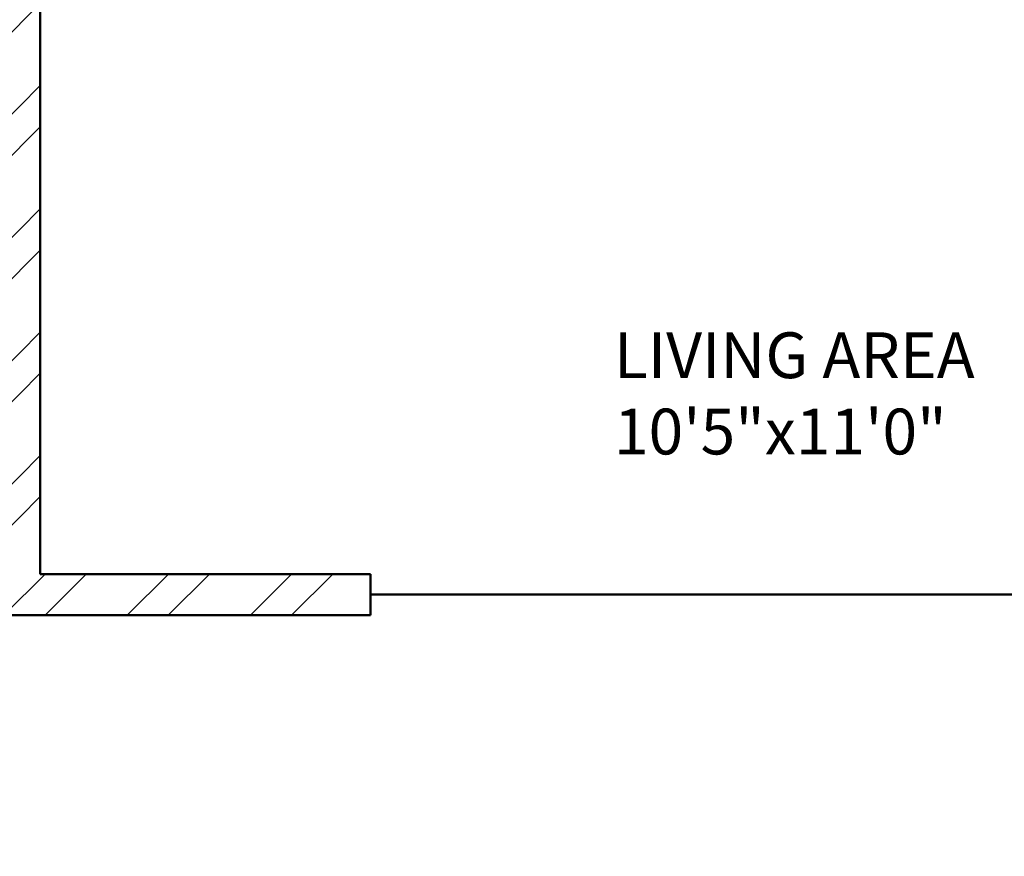
# Model space of a CAD drawing. Units: inches. Extents: x 1901 to 2863, y 888 to 2433.
# Tile 18 of 91: x 2157 to 2264, y 1549 to 1641. Entities that reach past the tile are written whole.
import ezdxf

# ---------------------------------------------------------------- set-up
doc = ezdxf.new("R2010")
doc.units = ezdxf.units.IN
for name, color, linetype, lineweight in [('A-AREA-IDEN', 7, 'Continuous', 18), ('A-WALL', 7, 'Continuous', 50), ('A-WALL-PATT', 8, 'Continuous', 13)]:
    doc.layers.add(name, color=color, linetype=linetype, lineweight=lineweight)
doc.styles.get("Standard").update_dxf_attribs({"font": 'arial.ttf'})

msp = doc.modelspace()

# ---------------------------------------------------------------- hatches: boundary and pattern name
at = {"layer": 'A-WALL-PATT'}
h = msp.add_hatch(dxfattribs=at)
h.set_pattern_fill('ANSI32', color=256)
h.paths.add_polyline_path([(2192.5, 2274.13), (2141.26, 2274.13), (2141.26, 2269.63), (2192.5, 2269.63)])
h.paths.add_polyline_path([(2259.93, 2274.13), (2216.5, 2274.13), (2216.5, 2269.63), (2255.43, 2269.63), (2255.43, 2214.63), (2250.81, 2214.63), (2250.81, 2210.13), (2259.93, 2210.13), (2259.93, 2215.13), (2271.76, 2215.13), (2271.76, 2217.38), (2271.76, 2219.63), (2259.93, 2219.63)])
h.paths.add_polyline_path([(2171.43, 2269.63), (2166.93, 2269.63), (2166.93, 2219.63), (2121.24, 2219.63), (2121.24, 2215.13), (2166.93, 2215.13), (2166.93, 2083.13), (2161.81, 2083.13), (2161.81, 2078.63), (2171.43, 2078.63), (2177, 2078.63), (2177, 2080.88), (2177, 2083.13), (2171.43, 2083.13), (2171.43, 2210.13), (2230.91, 2210.13), (2230.91, 2212.38), (2230.91, 2214.63), (2171.43, 2214.63)])
h.paths.add_polyline_path([(2117.26, 2274.13), (2089.43, 2274.13), (2089.43, 2219.63), (2081.14, 2219.63), (2081.14, 2215.13), (2089.43, 2215.13), (2098, 2215.13), (2098, 2217.38), (2098, 2219.63), (2093.93, 2219.63), (2093.93, 2269.63), (2117.26, 2269.63), (2117.26, 2271.88)])
h.paths.add_polyline_path([(2343.43, 2219.63), (2329.29, 2219.63), (2329.29, 2215.13), (2338.93, 2215.13), (2338.93, 2184.74), (2343.43, 2184.74)])
h.paths.add_polyline_path([(2338.93, 2083.13), (2329.29, 2083.13), (2208.97, 2083.13), (2208.97, 2078.63), (2338.93, 2078.63)])
h.paths.add_polyline_path([(2343.43, 2136.74), (2338.93, 2136.74), (2338.93, 1872.63), (2343.43, 1872.63)])
h.paths.add_polyline_path([(2343.43, 1863.63), (2397.68, 1863.63), (2397.68, 1821.63), (2384.14, 1821.63), (2384.14, 1812.63), (2418.33, 1812.63), (2418.33, 1817.13), (2418.33, 1821.63), (2406.68, 1821.63), (2406.68, 1863.63), (2459.5, 1863.63), (2459.5, 1821.63), (2447.14, 1821.63), (2447.14, 1812.63), (2459.5, 1812.63), (2468.5, 1812.63), (2468.5, 1872.63), (2394.43, 1872.63), (2334.43, 1872.63), (2334.43, 1812.63), (2343.43, 1812.63), (2353.25, 1812.63), (2353.25, 1821.63), (2343.43, 1821.63)])
h.paths.add_polyline_path([(2510.01, 1872.63), (2468.5, 1872.63), (2468.5, 1868.13), (2510.01, 1868.13)])
h.paths.add_polyline_path([(2514.01, 1817.13), (2468.5, 1817.13), (2468.5, 1812.63), (2482.11, 1812.63), (2482.11, 1800.61), (2486.61, 1800.61), (2486.61, 1812.63), (2514.01, 1812.63)])
h.paths.add_polyline_path([(2299.25, 1814.88), (2299.25, 1817.13), (2295.93, 1817.13), (2295.93, 1854.17), (2293.68, 1854.17), (2291.43, 1854.17), (2291.43, 1817.13), (2266.11, 1817.13), (2266.11, 1812.63), (2299.25, 1812.63)])
h.paths.add_polyline_path([(2218.11, 1817.13), (2206.46, 1817.13), (2171.43, 1817.13), (2171.43, 1949.13), (2190.1, 1949.13), (2190.1, 1953.63), (2163.47, 1953.63), (2163.47, 1949.13), (2166.93, 1949.13), (2166.93, 1817.13), (2114.3, 1817.13), (2114.3, 1812.63), (2218.11, 1812.63)])
h.paths.add_polyline_path([(2029.43, 1970.92), (2024.93, 1970.92), (2024.93, 1912.72), (2029.43, 1912.72)])
h.paths.add_polyline_path([(2132.3, 1953.63), (2113.93, 1953.63), (2113.93, 1975.89), (2111.68, 1975.89), (2109.43, 1975.89), (2109.43, 1953.63), (2029.43, 1953.63), (2029.43, 1949.13), (2132.3, 1949.13)])
h.paths.add_polyline_path([(2029.43, 1853.61), (2029.31, 1853.61), (2029.31, 1853.61), (2029.43, 1853.61), (2029.43, 1864.72), (2024.93, 1864.72), (2024.93, 1812.63), (2066.3, 1812.63), (2066.3, 1814.88), (2066.3, 1817.13), (2029.43, 1817.13)])
h.paths.add_polyline_path([(2122.93, 2010.09), (2120.68, 2010.09), (2118.43, 2010.09), (2118.43, 2006.13), (2029.43, 2006.13), (2029.43, 2001.63), (2109.43, 2001.63), (2109.43, 1998.04), (2113.93, 1998.04), (2113.93, 2001.63), (2122.93, 2001.63)])
h.paths.add_polyline_path([(2029.43, 2031.38), (2024.93, 2031.38), (2024.93, 1994.92), (2027.18, 1994.92), (2029.43, 1994.92)])
h.paths.add_polyline_path([(2029.43, 2136.74), (2024.93, 2136.74), (2024.93, 2067.38), (2027.18, 2067.38), (2029.43, 2067.38)])
h.paths.add_polyline_path([(2125.62, 2083.13), (2029.43, 2083.13), (2029.43, 2078.63), (2118.43, 2078.63), (2118.43, 2030.71), (2122.93, 2030.71), (2122.93, 2078.63), (2125.62, 2078.63)])
h.paths.add_polyline_path([(2029.43, 2215.13), (2040.47, 2215.13), (2040.47, 2217.38), (2040.47, 2219.63), (2024.93, 2219.63), (2024.93, 2184.74), (2029.43, 2184.74), (2029.43, 2187.78)])
h.paths.add_polyline_path([(2686.43, 2274.13), (2659.28, 2274.13), (2659.28, 2269.63), (2681.93, 2269.63), (2681.93, 2219.63), (2676.82, 2219.63), (2676.82, 2215.13), (2681.93, 2215.13), (2697.01, 2215.13), (2697.01, 2217.38), (2697.01, 2219.63), (2686.43, 2219.63)])
h.paths.add_polyline_path([(2609.93, 2269.63), (2635.28, 2269.63), (2635.28, 2274.13), (2571.43, 2274.13), (2571.43, 2269.63), (2605.43, 2269.63), (2605.43, 2214.63), (2549.1, 2214.63), (2549.1, 2210.13), (2605.43, 2210.13), (2605.43, 2083.13), (2601.01, 2083.13), (2601.01, 2080.88), (2601.01, 2078.63), (2609.93, 2078.63), (2616.16, 2078.63), (2616.16, 2080.88), (2616.16, 2083.13), (2609.93, 2083.13), (2609.93, 2215.13), (2651.46, 2215.13), (2651.46, 2217.38), (2651.46, 2219.63), (2609.93, 2219.63)])
h.paths.add_polyline_path([(2521.43, 2269.63), (2547.43, 2269.63), (2547.43, 2271.88), (2547.43, 2274.13), (2516.93, 2274.13), (2516.93, 2219.63), (2506.41, 2219.63), (2506.41, 2215.13), (2516.93, 2215.13), (2516.93, 2210.13), (2525.4, 2210.13), (2525.4, 2212.38), (2525.4, 2214.63), (2521.43, 2214.63)])
h.paths.add_polyline_path([(2456.01, 2219.63), (2439.43, 2219.63), (2439.43, 2187.89), (2443.93, 2187.89), (2443.93, 2215.13), (2456.01, 2215.13)])
h.paths.add_polyline_path([(2752.93, 2219.63), (2739.48, 2219.63), (2739.48, 2215.13), (2748.43, 2215.13), (2748.43, 2187.89), (2752.93, 2187.89)])
h.paths.add_polyline_path([(2752.93, 2139.89), (2748.43, 2139.89), (2748.43, 2083.13), (2648.42, 2083.13), (2648.42, 2078.63), (2654.93, 2078.63), (2654.93, 2039.44), (2659.43, 2039.44), (2659.43, 2078.63), (2748.43, 2078.63), (2748.43, 2063.43), (2752.93, 2063.43)])
h.paths.add_polyline_path([(2752.93, 2010.63), (2659.43, 2010.63), (2659.43, 2015.65), (2654.93, 2015.65), (2654.93, 2010.63), (2605.43, 2010.63), (2605.43, 1920.97), (2609.93, 1920.97), (2609.93, 2006.13), (2748.43, 2006.13), (2748.43, 1982.47), (2752.93, 1982.47)])
h.paths.add_polyline_path([(2752.93, 2027.43), (2748.43, 2027.43), (2748.43, 2010.63), (2752.93, 2010.63)])
h.paths.add_polyline_path([(2748.43, 1886.13), (2609.93, 1886.13), (2609.93, 1889.72), (2605.43, 1889.72), (2605.43, 1861.26), (2609.93, 1861.26), (2609.93, 1881.63), (2748.43, 1881.63)])
h.paths.add_polyline_path([(2456.86, 2228.83), (2498.4, 2228.83), (2498.4, 2247.49), (2456.86, 2247.49)], flags=9)
h.paths.add_polyline_path([(2038.6, 2237.42), (2080.17, 2237.42), (2080.17, 2256.08), (2038.6, 2256.08)], flags=9)
h.paths.add_polyline_path([(2292.01, 1062.39), (2539.93, 1062.39), (2539.93, 1099.49), (2292.01, 1099.49)], flags=9)
h.paths.add_polyline_path([(2424.91, 1832.25), (2448.51, 1832.25), (2448.51, 1846.68), (2424.91, 1846.68)], flags=25)
h.paths.add_polyline_path([(2359.08, 1832.25), (2382.68, 1832.25), (2382.68, 1846.68), (2359.08, 1846.68)], flags=25)
h.paths.add_polyline_path([(2352.9, 1684.8), (2367.54, 1684.8), (2367.54, 1697.17), (2352.9, 1697.17)], flags=9)
h.paths.add_polyline_path([(2079.29, 1755.83), (2169.02, 1755.83), (2169.02, 1774.37), (2079.29, 1774.37)], flags=9)
h.paths.add_polyline_path([(2404.09, 1373.86), (2404.09, 1463.59), (2385.54, 1463.59), (2385.54, 1373.86)], flags=9)
h.paths.add_polyline_path([(2268.09, 2236.37), (2309.64, 2236.37), (2309.64, 2255.03), (2268.09, 2255.03)], flags=9)
h.paths.add_polyline_path([(2575.96, 1700.95), (2665.7, 1700.95), (2665.7, 1719.5), (2575.96, 1719.5)], flags=9)
h.paths.add_polyline_path([(2302.96, 1878.47), (2329.52, 1878.47), (2329.52, 1888.78), (2302.96, 1888.78)], flags=9)
h.paths.add_polyline_path([(2097.42, 2240.58), (2126.57, 2240.58), (2126.57, 2259.23), (2097.42, 2259.23)], flags=9)
h.paths.add_polyline_path([(2208.72, 2246.12), (2237.88, 2246.12), (2237.88, 2264.78), (2208.72, 2264.78)], flags=9)
h.paths.add_polyline_path([(2038.15, 1925.96), (2076.99, 1925.96), (2076.99, 1944.62), (2038.15, 1944.62)], flags=9)
h.paths.add_polyline_path([(2239.14, 1926.67), (2288.46, 1926.67), (2288.46, 1945.33), (2239.14, 1945.33)], flags=9)
h.paths.add_polyline_path([(2175.43, 2007.33), (2212.36, 2007.33), (2212.36, 2025.99), (2175.43, 2025.99)], flags=9)
h.paths.add_polyline_path([(2225.03, 2091.79), (2263.87, 2091.79), (2263.87, 2110.45), (2225.03, 2110.45)], flags=9)
h.paths.add_polyline_path([(2035.4, 2098.48), (2074.24, 2098.48), (2074.24, 2117.14), (2035.4, 2117.14)], flags=9)
h.paths.add_polyline_path([(2050.1, 2029.21), (2083.26, 2029.21), (2083.26, 2047.87), (2050.1, 2047.87)], flags=9)
h.paths.add_polyline_path([(2069.68, 1956.72), (2098.83, 1956.72), (2098.83, 1975.38), (2069.68, 1975.38)], flags=25)
h.paths.add_polyline_path([(2328.62, 1753.34), (2361.66, 1753.34), (2361.66, 1771.99), (2328.62, 1771.99)], flags=9)
h.paths.add_polyline_path([(2395.16, 2060.89), (2395.16, 2140.65), (2378.68, 2140.65), (2378.68, 2060.89)], flags=9)
h.paths.add_polyline_path([(2463.73, 2059.02), (2492.89, 2059.02), (2492.89, 2077.68), (2463.73, 2077.68)], flags=9)
h.paths.add_polyline_path([(2458.03, 2181.54), (2496.87, 2181.54), (2496.87, 2200.19), (2458.03, 2200.19)], flags=9)
h.paths.add_polyline_path([(2527.58, 2243.07), (2556.73, 2243.07), (2556.73, 2261.73), (2527.58, 2261.73)], flags=9)
h.paths.add_polyline_path([(2694.46, 2232.77), (2736.03, 2232.77), (2736.03, 2251.42), (2694.46, 2251.42)], flags=9)
h.paths.add_polyline_path([(2637.82, 2249.22), (2666.98, 2249.22), (2666.98, 2267.88), (2637.82, 2267.88)], flags=9)
h.paths.add_polyline_path([(2623.69, 2183.54), (2662.53, 2183.54), (2662.53, 2202.2), (2623.69, 2202.2)], flags=9)
h.paths.add_polyline_path([(2691.97, 2021.5), (2725.12, 2021.5), (2725.12, 2040.16), (2691.97, 2040.16)], flags=9)
h.paths.add_polyline_path([(2621.04, 1975.91), (2662.34, 1975.91), (2662.34, 1994.57), (2621.04, 1994.57)], flags=25)
h.paths.add_polyline_path([(2479.03, 1927.62), (2519.84, 1927.62), (2519.84, 1946.28), (2479.03, 1946.28)], flags=9)
h.paths.add_polyline_path([(2670.94, 1849.08), (2716.01, 1849.08), (2716.01, 1867.73), (2670.94, 1867.73)], flags=9)
h.paths.add_polyline_path([(2523.61, 1782.96), (2550.17, 1782.96), (2550.17, 1793.26), (2523.61, 1793.26)], flags=9)
h.paths.add_polyline_path([(2450.84, 1207.33), (2492.39, 1207.33), (2492.39, 1225.99), (2450.84, 1225.99)], flags=9)
h.paths.add_polyline_path([(2527.75, 1203.84), (2556.91, 1203.84), (2556.91, 1222.5), (2527.75, 1222.5)], flags=9)
h.paths.add_polyline_path([(2639.11, 1207.2), (2668.27, 1207.2), (2668.27, 1225.86), (2639.11, 1225.86)], flags=9)
h.paths.add_polyline_path([(2692.59, 1218.97), (2734.17, 1218.97), (2734.17, 1237.62), (2692.59, 1237.62)], flags=9)
h.paths.add_polyline_path([(2669.27, 1366.33), (2708.11, 1366.33), (2708.11, 1384.99), (2669.27, 1384.99)], flags=9)
h.paths.add_polyline_path([(2463.31, 1358.03), (2502.15, 1358.03), (2502.15, 1376.69), (2463.31, 1376.69)], flags=9)
h.paths.add_polyline_path([(2494.72, 1449.96), (2531.65, 1449.96), (2531.65, 1468.62), (2494.72, 1468.62)], flags=9)
h.paths.add_polyline_path([(2675.57, 1422.16), (2708.72, 1422.16), (2708.72, 1440.81), (2675.57, 1440.81)], flags=9)
h.paths.add_polyline_path([(2685.63, 1493.89), (2714.79, 1493.89), (2714.79, 1512.55), (2685.63, 1512.55)], flags=9)
h.paths.add_polyline_path([(2686.8, 1529.91), (2725.65, 1529.91), (2725.65, 1548.57), (2686.8, 1548.57)], flags=9)
h.paths.add_polyline_path([(2503.65, 1537.99), (2552.97, 1537.99), (2552.97, 1556.65), (2503.65, 1556.65)], flags=9)
h.paths.add_polyline_path([(2291.71, 1643.5), (2318.28, 1643.5), (2318.28, 1653.81), (2291.71, 1653.81)], flags=9)
h.paths.add_polyline_path([(2450.63, 1610.52), (2477.19, 1610.52), (2477.19, 1620.82), (2450.63, 1620.82)], flags=9)
h.paths.add_polyline_path([(2359.99, 1551.81), (2422.25, 1551.81), (2422.25, 1562.12), (2359.99, 1562.12)], flags=9)
h.paths.add_polyline_path([(2280.11, 1249.01), (2321.65, 1249.01), (2321.65, 1267.66), (2280.11, 1267.66)], flags=9)
h.paths.add_polyline_path([(2164.06, 1274.23), (2193.22, 1274.23), (2193.22, 1292.89), (2164.06, 1292.89)], flags=9)
h.paths.add_polyline_path([(2118.21, 1277.69), (2151.25, 1277.69), (2151.25, 1296.35), (2118.21, 1296.35)], flags=9)
h.paths.add_polyline_path([(2031.95, 1268.53), (2073.52, 1268.53), (2073.52, 1287.19), (2031.95, 1287.19)], flags=9)
h.paths.add_polyline_path([(2050.2, 1409.08), (2089.04, 1409.08), (2089.04, 1427.74), (2050.2, 1427.74)], flags=9)
h.paths.add_polyline_path([(2243.74, 1421.03), (2282.58, 1421.03), (2282.58, 1439.69), (2243.74, 1439.69)], flags=9)
h.paths.add_polyline_path([(2190.75, 1509.77), (2231.56, 1509.77), (2231.56, 1528.43), (2190.75, 1528.43)], flags=9)
h.paths.add_polyline_path([(2058.39, 1475.42), (2091.55, 1475.42), (2091.55, 1494.07), (2058.39, 1494.07)], flags=9)
h.paths.add_polyline_path([(2062.45, 1553.09), (2091.6, 1553.09), (2091.6, 1571.75), (2062.45, 1571.75)], flags=9)
h.paths.add_polyline_path([(2219.52, 1590.37), (2266.15, 1590.37), (2266.15, 1609.02), (2219.52, 1609.02)], flags=9)
h.paths.add_polyline_path([(2041.07, 1584.19), (2079.91, 1584.19), (2079.91, 1602.85), (2041.07, 1602.85)], flags=9)
h = msp.add_hatch(dxfattribs=at)
h.set_pattern_fill('ANSI32', color=256)
h.paths.add_polyline_path([(2443.93, 2139.89), (2439.43, 2139.89), (2439.43, 2069.35), (2441.68, 2069.35), (2443.93, 2069.35), (2443.93, 2078.63), (2521.93, 2078.63), (2521.93, 2075.07), (2524.18, 2075.07), (2526.43, 2075.07), (2526.43, 2078.63), (2571.75, 2078.63), (2571.75, 2080.88), (2571.75, 2083.13), (2443.93, 2083.13)])
h.paths.add_polyline_path([(2526.43, 2054.63), (2524.18, 2054.63), (2521.93, 2054.63), (2521.93, 2030.63), (2443.93, 2030.63), (2443.93, 2045.35), (2439.43, 2045.35), (2439.43, 1983.87), (2443.93, 1983.87), (2443.93, 2026.13), (2521.93, 2026.13), (2526.43, 2026.13)])
h.paths.add_polyline_path([(2443.93, 1923.87), (2439.43, 1923.87), (2439.43, 1872.63), (2443.93, 1872.63)])
h.paths.add_polyline_path([(2636.23, 1766.13), (2609.93, 1766.13), (2609.93, 1779.79), (2605.43, 1779.79), (2605.43, 1766.13), (2486.61, 1766.13), (2486.61, 1770.67), (2482.11, 1770.67), (2482.11, 1766.13), (2482.11, 1761.63), (2636.23, 1761.63), (2636.23, 1763.88)])
h.paths.add_polyline_path([(2519.54, 1663.38), (2519.54, 1665.63), (2494.93, 1665.63), (2481.83, 1665.63), (2481.83, 1663.38), (2481.83, 1661.13), (2490.43, 1661.13), (2490.43, 1640.16), (2494.93, 1640.16), (2494.93, 1661.13), (2519.54, 1661.13)])
h.paths.add_polyline_path([(2443.93, 1712.13), (2443.93, 1716.63), (2414.46, 1716.63), (2414.46, 1712.13), (2439.43, 1712.13), (2439.43, 1545.51), (2443.93, 1545.51), (2443.93, 1661.13), (2448.47, 1661.13), (2448.47, 1665.63), (2443.93, 1665.63)])
h.paths.add_polyline_path([(2343.43, 1712.13), (2365.52, 1712.13), (2365.52, 1714.38), (2365.52, 1716.63), (2333.87, 1716.63), (2333.87, 1714.38), (2333.87, 1712.13), (2338.93, 1712.13), (2338.93, 1575.63), (2338.93, 1545.51), (2343.43, 1545.51), (2343.43, 1547.51), (2343.43, 1580.13)])
h.paths.add_polyline_path([(2752.93, 1665.63), (2579.54, 1665.63), (2579.54, 1661.13), (2615.93, 1661.13), (2615.93, 1529.13), (2598.93, 1529.13), (2598.93, 1524.63), (2623.13, 1524.63), (2623.13, 1526.88), (2623.13, 1529.13), (2620.43, 1529.13), (2620.43, 1661.13), (2748.43, 1661.13), (2748.43, 1633.5), (2752.93, 1633.5)])
h.paths.add_polyline_path([(2752.93, 1419.93), (2748.43, 1419.93), (2748.43, 1400.13), (2659.43, 1400.13), (2659.43, 1444.33), (2657.18, 1444.33), (2654.93, 1444.33), (2654.93, 1400.13), (2643.65, 1400.13), (2643.65, 1395.63), (2748.43, 1395.63), (2748.43, 1364.04), (2752.93, 1364.04)])
h.paths.add_polyline_path([(2752.93, 1492.88), (2748.43, 1492.88), (2748.43, 1476.63), (2667.43, 1476.63), (2667.43, 1479.71), (2665.18, 1479.71), (2662.93, 1479.71), (2662.93, 1476.63), (2654.93, 1476.63), (2654.93, 1469.54), (2659.43, 1469.54), (2659.43, 1472.13), (2748.43, 1472.13), (2748.43, 1455.93), (2752.93, 1455.93)])
h.paths.add_polyline_path([(2752.93, 1304.04), (2748.43, 1304.04), (2748.43, 1263.63), (2738.66, 1263.63), (2738.66, 1259.13), (2752.93, 1259.13)])
h.paths.add_polyline_path([(2685.93, 1259.13), (2695.49, 1259.13), (2695.49, 1261.38), (2695.49, 1263.63), (2677.84, 1263.63), (2677.84, 1261.38), (2677.84, 1259.13), (2681.43, 1259.13), (2681.43, 1203.63), (2653.28, 1203.63), (2653.28, 1199.13), (2685.93, 1199.13), (2685.93, 1203.63)])
h.paths.add_polyline_path([(2609.43, 1395.63), (2611.85, 1395.63), (2611.85, 1400.13), (2598.89, 1400.13), (2598.89, 1397.88), (2598.89, 1395.63), (2604.93, 1395.63), (2604.93, 1268.13), (2554.73, 1268.13), (2554.73, 1265.88), (2554.73, 1263.63), (2604.93, 1263.63), (2604.93, 1203.63), (2571.31, 1203.63), (2571.31, 1199.13), (2604.93, 1199.13), (2629.28, 1199.13), (2629.28, 1201.38), (2629.28, 1203.63), (2609.43, 1203.63), (2609.43, 1258.63), (2609.43, 1259.13), (2654.8, 1259.13), (2654.8, 1263.63), (2609.43, 1263.63)])
h.paths.add_polyline_path([(2443.93, 1304.04), (2439.43, 1304.04), (2439.43, 1259.13), (2443.93, 1259.13), (2456.16, 1259.13), (2456.16, 1261.38), (2456.16, 1263.63), (2443.93, 1263.63)])
h.paths.add_polyline_path([(2525.43, 1263.63), (2531.78, 1263.63), (2531.78, 1268.13), (2520.93, 1268.13), (2520.93, 1263.63), (2511.41, 1263.63), (2511.41, 1259.13), (2520.93, 1259.13), (2520.93, 1199.13), (2547.31, 1199.13), (2547.31, 1201.38), (2547.31, 1203.63), (2525.43, 1203.63)])
h.paths.add_polyline_path([(2443.93, 1434.84), (2439.43, 1434.84), (2439.43, 1364.04), (2441.68, 1364.04), (2443.93, 1364.04)])
h.paths.add_polyline_path([(2567.13, 1400.13), (2443.93, 1400.13), (2443.93, 1395.63), (2567.13, 1395.63)])
h.paths.add_polyline_path([(2443.93, 1545.51), (2439.43, 1545.51), (2439.43, 1494.84), (2443.93, 1494.84)])
h.paths.add_polyline_path([(2494.93, 1553.35), (2492.68, 1553.35), (2490.43, 1553.35), (2490.43, 1524.63), (2494.93, 1524.63), (2525.94, 1524.63), (2525.94, 1526.88), (2525.94, 1529.13), (2494.93, 1529.13)])
h.paths.add_polyline_path([(2752.93, 1573.5), (2748.43, 1573.5), (2748.43, 1529.13), (2657.76, 1529.13), (2657.76, 1524.63), (2662.93, 1524.63), (2662.93, 1498.63), (2667.43, 1498.63), (2667.43, 1524.63), (2748.43, 1524.63), (2748.43, 1516.88), (2752.93, 1516.88)])
h.paths.add_polyline_path([(2038.6, 2237.42), (2080.17, 2237.42), (2080.17, 2256.08), (2038.6, 2256.08)], flags=9)
h.paths.add_polyline_path([(2292.01, 1062.39), (2539.93, 1062.39), (2539.93, 1099.49), (2292.01, 1099.49)], flags=9)
h.paths.add_polyline_path([(2424.91, 1832.25), (2448.51, 1832.25), (2448.51, 1846.68), (2424.91, 1846.68)], flags=9)
h.paths.add_polyline_path([(2359.08, 1832.25), (2382.68, 1832.25), (2382.68, 1846.68), (2359.08, 1846.68)], flags=9)
h.paths.add_polyline_path([(2352.9, 1684.8), (2367.54, 1684.8), (2367.54, 1697.17), (2352.9, 1697.17)], flags=9)
h.paths.add_polyline_path([(2079.29, 1755.83), (2169.02, 1755.83), (2169.02, 1774.37), (2079.29, 1774.37)], flags=9)
h.paths.add_polyline_path([(2404.09, 1373.86), (2404.09, 1463.59), (2385.54, 1463.59), (2385.54, 1373.86)], flags=9)
h.paths.add_polyline_path([(2268.09, 2236.37), (2309.64, 2236.37), (2309.64, 2255.03), (2268.09, 2255.03)], flags=9)
h.paths.add_polyline_path([(2575.96, 1700.95), (2665.7, 1700.95), (2665.7, 1719.5), (2575.96, 1719.5)], flags=9)
h.paths.add_polyline_path([(2302.96, 1878.47), (2329.52, 1878.47), (2329.52, 1888.78), (2302.96, 1888.78)], flags=9)
h.paths.add_polyline_path([(2097.42, 2240.58), (2126.57, 2240.58), (2126.57, 2259.23), (2097.42, 2259.23)], flags=9)
h.paths.add_polyline_path([(2208.72, 2246.12), (2237.88, 2246.12), (2237.88, 2264.78), (2208.72, 2264.78)], flags=9)
h.paths.add_polyline_path([(2038.15, 1925.96), (2076.99, 1925.96), (2076.99, 1944.62), (2038.15, 1944.62)], flags=9)
h.paths.add_polyline_path([(2239.14, 1926.67), (2288.46, 1926.67), (2288.46, 1945.33), (2239.14, 1945.33)], flags=9)
h.paths.add_polyline_path([(2175.43, 2007.33), (2212.36, 2007.33), (2212.36, 2025.99), (2175.43, 2025.99)], flags=9)
h.paths.add_polyline_path([(2225.03, 2091.79), (2263.87, 2091.79), (2263.87, 2110.45), (2225.03, 2110.45)], flags=9)
h.paths.add_polyline_path([(2035.4, 2098.48), (2074.24, 2098.48), (2074.24, 2117.14), (2035.4, 2117.14)], flags=9)
h.paths.add_polyline_path([(2050.1, 2029.21), (2083.26, 2029.21), (2083.26, 2047.87), (2050.1, 2047.87)], flags=9)
h.paths.add_polyline_path([(2069.68, 1956.72), (2098.83, 1956.72), (2098.83, 1975.38), (2069.68, 1975.38)], flags=9)
h.paths.add_polyline_path([(2328.62, 1753.34), (2361.66, 1753.34), (2361.66, 1771.99), (2328.62, 1771.99)], flags=9)
h.paths.add_polyline_path([(2395.16, 2060.89), (2395.16, 2140.65), (2378.68, 2140.65), (2378.68, 2060.89)], flags=9)
h.paths.add_polyline_path([(2463.73, 2059.02), (2492.89, 2059.02), (2492.89, 2077.68), (2463.73, 2077.68)], flags=9)
h.paths.add_polyline_path([(2458.03, 2181.54), (2496.87, 2181.54), (2496.87, 2200.19), (2458.03, 2200.19)], flags=9)
h.paths.add_polyline_path([(2456.86, 2228.83), (2498.4, 2228.83), (2498.4, 2247.49), (2456.86, 2247.49)], flags=9)
h.paths.add_polyline_path([(2527.58, 2243.07), (2556.73, 2243.07), (2556.73, 2261.73), (2527.58, 2261.73)], flags=9)
h.paths.add_polyline_path([(2694.46, 2232.77), (2736.03, 2232.77), (2736.03, 2251.42), (2694.46, 2251.42)], flags=9)
h.paths.add_polyline_path([(2637.82, 2249.22), (2666.98, 2249.22), (2666.98, 2267.88), (2637.82, 2267.88)], flags=9)
h.paths.add_polyline_path([(2623.69, 2183.54), (2662.53, 2183.54), (2662.53, 2202.2), (2623.69, 2202.2)], flags=9)
h.paths.add_polyline_path([(2691.97, 2021.5), (2725.12, 2021.5), (2725.12, 2040.16), (2691.97, 2040.16)], flags=9)
h.paths.add_polyline_path([(2621.04, 1975.91), (2662.34, 1975.91), (2662.34, 1994.57), (2621.04, 1994.57)], flags=9)
h.paths.add_polyline_path([(2479.03, 1927.62), (2519.84, 1927.62), (2519.84, 1946.28), (2479.03, 1946.28)], flags=9)
h.paths.add_polyline_path([(2670.94, 1849.08), (2716.01, 1849.08), (2716.01, 1867.73), (2670.94, 1867.73)], flags=9)
h.paths.add_polyline_path([(2523.61, 1782.96), (2550.17, 1782.96), (2550.17, 1793.26), (2523.61, 1793.26)], flags=9)
h.paths.add_polyline_path([(2450.84, 1207.33), (2492.39, 1207.33), (2492.39, 1225.99), (2450.84, 1225.99)], flags=9)
h.paths.add_polyline_path([(2527.75, 1203.84), (2556.91, 1203.84), (2556.91, 1222.5), (2527.75, 1222.5)], flags=9)
h.paths.add_polyline_path([(2639.11, 1207.2), (2668.27, 1207.2), (2668.27, 1225.86), (2639.11, 1225.86)], flags=9)
h.paths.add_polyline_path([(2692.59, 1218.97), (2734.17, 1218.97), (2734.17, 1237.62), (2692.59, 1237.62)], flags=9)
h.paths.add_polyline_path([(2669.27, 1366.33), (2708.11, 1366.33), (2708.11, 1384.99), (2669.27, 1384.99)], flags=25)
h.paths.add_polyline_path([(2463.31, 1358.03), (2502.15, 1358.03), (2502.15, 1376.69), (2463.31, 1376.69)], flags=9)
h.paths.add_polyline_path([(2494.72, 1449.96), (2531.65, 1449.96), (2531.65, 1468.62), (2494.72, 1468.62)], flags=9)
h.paths.add_polyline_path([(2675.57, 1422.16), (2708.72, 1422.16), (2708.72, 1440.81), (2675.57, 1440.81)], flags=25)
h.paths.add_polyline_path([(2685.63, 1493.89), (2714.79, 1493.89), (2714.79, 1512.55), (2685.63, 1512.55)], flags=9)
h.paths.add_polyline_path([(2686.8, 1529.91), (2725.65, 1529.91), (2725.65, 1548.57), (2686.8, 1548.57)], flags=25)
h.paths.add_polyline_path([(2503.65, 1537.99), (2552.97, 1537.99), (2552.97, 1556.65), (2503.65, 1556.65)], flags=9)
h.paths.add_polyline_path([(2291.71, 1643.5), (2318.28, 1643.5), (2318.28, 1653.81), (2291.71, 1653.81)], flags=9)
h.paths.add_polyline_path([(2450.63, 1610.52), (2477.19, 1610.52), (2477.19, 1620.82), (2450.63, 1620.82)], flags=9)
h.paths.add_polyline_path([(2359.99, 1551.81), (2422.25, 1551.81), (2422.25, 1562.12), (2359.99, 1562.12)], flags=9)
h.paths.add_polyline_path([(2280.11, 1249.01), (2321.65, 1249.01), (2321.65, 1267.66), (2280.11, 1267.66)], flags=9)
h.paths.add_polyline_path([(2164.06, 1274.23), (2193.22, 1274.23), (2193.22, 1292.89), (2164.06, 1292.89)], flags=9)
h.paths.add_polyline_path([(2118.21, 1277.69), (2151.25, 1277.69), (2151.25, 1296.35), (2118.21, 1296.35)], flags=9)
h.paths.add_polyline_path([(2031.95, 1268.53), (2073.52, 1268.53), (2073.52, 1287.19), (2031.95, 1287.19)], flags=9)
h.paths.add_polyline_path([(2050.2, 1409.08), (2089.04, 1409.08), (2089.04, 1427.74), (2050.2, 1427.74)], flags=9)
h.paths.add_polyline_path([(2243.74, 1421.03), (2282.58, 1421.03), (2282.58, 1439.69), (2243.74, 1439.69)], flags=9)
h.paths.add_polyline_path([(2190.75, 1509.77), (2231.56, 1509.77), (2231.56, 1528.43), (2190.75, 1528.43)], flags=9)
h.paths.add_polyline_path([(2058.39, 1475.42), (2091.55, 1475.42), (2091.55, 1494.07), (2058.39, 1494.07)], flags=9)
h.paths.add_polyline_path([(2062.45, 1553.09), (2091.6, 1553.09), (2091.6, 1571.75), (2062.45, 1571.75)], flags=9)
h.paths.add_polyline_path([(2219.52, 1590.37), (2266.15, 1590.37), (2266.15, 1609.02), (2219.52, 1609.02)], flags=9)
h.paths.add_polyline_path([(2041.07, 1584.19), (2079.91, 1584.19), (2079.91, 1602.85), (2041.07, 1602.85)], flags=9)
h = msp.add_hatch(dxfattribs=at)
h.set_pattern_fill('ANSI32', color=256)
h.paths.add_polyline_path([(2182.93, 1716.63), (2024.93, 1716.63), (2024.93, 1681.7), (2029.33, 1681.7), (2029.33, 1712.13), (2154.33, 1712.13), (2154.33, 1580.13), (2148.52, 1580.13), (2148.52, 1577.88), (2148.52, 1575.63), (2194.93, 1575.63), (2194.93, 1580.13), (2158.83, 1580.13), (2158.83, 1712.13), (2182.93, 1712.13)])
h.paths.add_polyline_path([(2301.07, 1716.63), (2242.93, 1716.63), (2242.93, 1712.13), (2283.83, 1712.13), (2283.83, 1685.54), (2288.33, 1685.54), (2288.33, 1712.13), (2301.07, 1712.13)])
h.paths.add_polyline_path([(2288.33, 1600.41), (2286.08, 1600.41), (2283.83, 1600.41), (2283.83, 1580.13), (2270.6, 1580.13), (2270.6, 1575.63), (2288.33, 1575.63)])
h.paths.add_polyline_path([(2295.93, 1953.63), (2271.45, 1953.63), (2271.45, 1949.13), (2291.43, 1949.13), (2291.43, 1941.24), (2295.93, 1941.24)])
h.paths.add_polyline_path([(2098.38, 1244.13), (2082.33, 1244.13), (2082.33, 1302.13), (2086.52, 1302.13), (2086.52, 1306.63), (2067.46, 1306.63), (2067.46, 1302.13), (2077.83, 1302.13), (2077.83, 1239.63), (2098.38, 1239.63), (2098.38, 1241.88)])
h.paths.add_polyline_path([(2217.31, 1306.63), (2158.83, 1306.63), (2158.83, 1451.63), (2162.72, 1451.63), (2162.72, 1453.88), (2162.72, 1456.13), (2154.33, 1456.13), (2154.33, 1443.13), (2151.91, 1443.13), (2151.91, 1438.63), (2154.33, 1438.63), (2154.33, 1306.63), (2109.31, 1306.63), (2109.31, 1304.38), (2109.31, 1302.13), (2154.33, 1302.13), (2154.33, 1244.13), (2122.38, 1244.13), (2122.38, 1239.63), (2154.33, 1239.63), (2154.33, 1223.63), (2163.33, 1223.63), (2181.01, 1223.63), (2181.01, 1225.88), (2181.01, 1228.13), (2163.33, 1228.13), (2163.33, 1258.22), (2158.83, 1258.22), (2158.83, 1302.13), (2217.31, 1302.13)])
h.paths.add_polyline_path([(2259.99, 1306.63), (2238.3, 1306.63), (2238.3, 1304.38), (2238.3, 1302.13), (2242.83, 1302.13), (2242.83, 1228.13), (2205.01, 1228.13), (2205.01, 1223.63), (2247.33, 1223.63), (2247.33, 1302.13), (2259.99, 1302.13), (2259.99, 1304.38)])
h.paths.add_polyline_path([(2343.43, 1361.7), (2338.93, 1361.7), (2338.93, 1306.63), (2322.38, 1306.63), (2322.38, 1302.13), (2343.43, 1302.13)])
h.paths.add_polyline_path([(2343.43, 1470.4), (2338.93, 1470.4), (2338.93, 1456.13), (2193.73, 1456.13), (2193.73, 1453.88), (2193.73, 1451.63), (2338.93, 1451.63), (2338.93, 1421.7), (2343.43, 1421.7)])
h.paths.add_polyline_path([(2343.43, 1545.51), (2338.93, 1545.51), (2338.93, 1530.4), (2343.43, 1530.4)])
h.paths.add_polyline_path([(2029.33, 1466.83), (2024.93, 1466.83), (2024.93, 1409.82), (2029.33, 1409.82)])
h.paths.add_polyline_path([(2122.84, 1440.88), (2122.84, 1443.13), (2121.83, 1443.13), (2121.83, 1498.18), (2119.58, 1498.18), (2117.33, 1498.18), (2117.33, 1443.13), (2029.33, 1443.13), (2029.33, 1438.63), (2122.84, 1438.63)])
h.paths.add_polyline_path([(2029.33, 1543.05), (2024.93, 1543.05), (2024.93, 1502.83), (2029.33, 1502.83)])
h.paths.add_polyline_path([(2029.33, 1621.7), (2024.93, 1621.7), (2024.93, 1567.05), (2027.13, 1567.05), (2029.33, 1567.05), (2029.33, 1575.63), (2109.33, 1575.63), (2109.33, 1554.71), (2113.83, 1554.71), (2113.83, 1575.63), (2115.8, 1575.63), (2115.8, 1577.88), (2115.8, 1580.13), (2029.33, 1580.13)])
h.paths.add_polyline_path([(2121.83, 1527.63), (2117.33, 1527.63), (2113.83, 1527.63), (2113.83, 1533.01), (2111.58, 1533.01), (2109.33, 1533.01), (2109.33, 1527.63), (2029.33, 1527.63), (2029.33, 1523.13), (2117.33, 1523.13), (2117.33, 1519.43), (2121.83, 1519.43)])
h.paths.add_polyline_path([(2029.33, 1349.82), (2024.93, 1349.82), (2024.93, 1302.13), (2036.28, 1302.13), (2036.28, 1306.63), (2029.33, 1306.63)])

# ---------------------------------------------------------------- linework, layer by layer
at = {"layer": 'A-WALL'}
for p, q in [((2158.83, 1712.13), (2158.83, 1580.13)), ((2194.93, 1580.13), (2158.83, 1580.13)), ((2194.93, 1580.13), (2194.93, 1575.63)), ((2270.6, 1577.88), (2194.93, 1577.88)), ((2194.93, 1575.63), (2148.52, 1575.63))]:
    msp.add_line(p, q, dxfattribs=at)

# ---------------------------------------------------------------- texts
at = {"layer": 'A-AREA-IDEN', "insert": (2221.53, 1606.53), "char_height": 5, "attachment_point": 1}
msp.add_mtext_dynamic_manual_height_columns('LIVING AREA\\P10\'5"x11\'0"', width=154.2094, gutter_width=12.5, heights=[0], dxfattribs=at)

doc.saveas('drawing.dxf')
